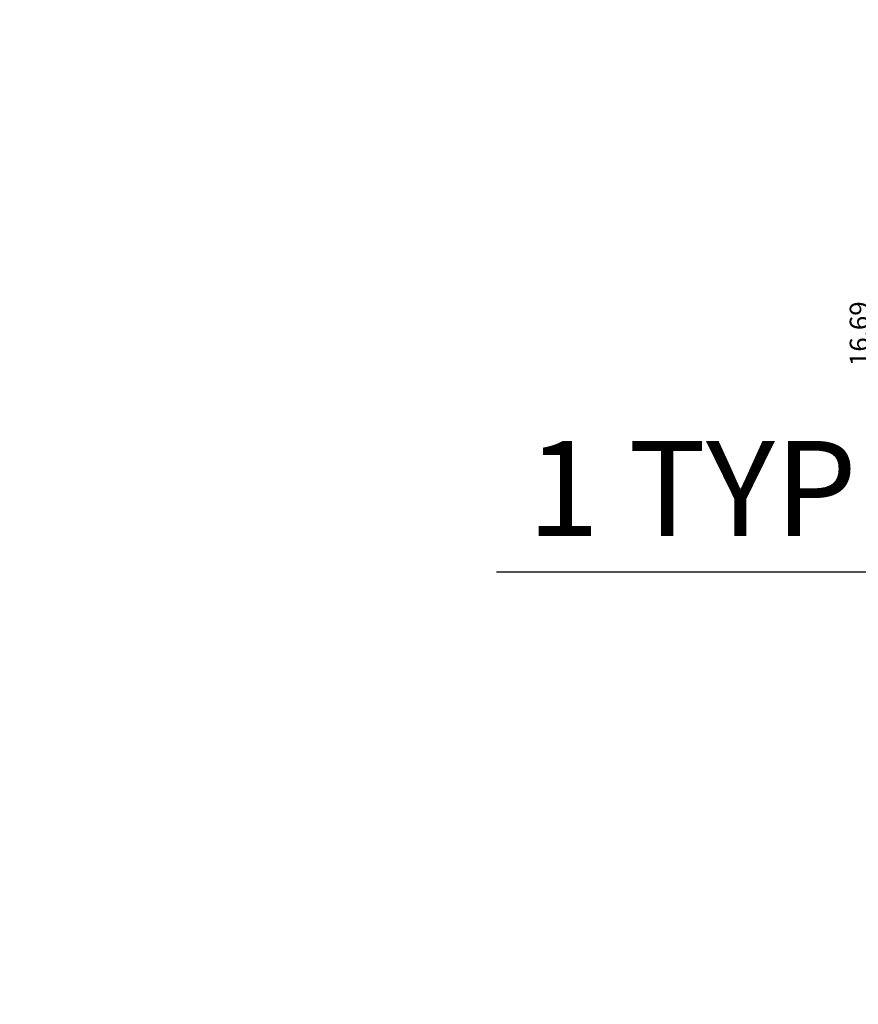
# Model space of a CAD drawing. Units: metres. Extents: x 1246 to 2549, y 2050 to 4184.
# Tile 2 of 6: x 1246 to 1268, y 2074 to 2100. Entities that reach past the tile are written whole.
import ezdxf

# ---------------------------------------------------------------- set-up
doc = ezdxf.new("R2010")
doc.units = ezdxf.units.M
doc.layers.add('A-ANNO-DIMS', color=2, linetype='Continuous', lineweight=18)
doc.styles.get("Standard").update_dxf_attribs({"font": 'arial.ttf'})
doc.dimstyles.new('ISO-25', dxfattribs={"dimtxt": 2.5, "dimasz": 2.5, "dimexe": 1.25, "dimexo": 0.625, "dimtad": 1, "dimtxsty": 'Standard', "dimcen": 2.5, "dimadec": 0, "dimazin": 0, "dimtfac": 1, "dimtmove": 0, "dimatfit": 3, "dimfxl": 1, "dimarcsym": 0})

# ---------------------------------------------------------------- blocks, each defined once
blk = doc.blocks.new('*D2')
at = {"layer": 'A-ANNO-DIMS', "color": 0, "lineweight": -2, "transparency": 16777216}
for p, q in [((1272.709, 2100.209), (1270.53, 2100.209)), ((1271.78, 2097.709), (1271.78, 2086.022)), ((1272.709, 2083.522), (1270.53, 2083.522))]:
    blk.add_line(p, q, dxfattribs=at)
at = {"layer": 'A-ANNO-DIMS', "color": 0, "transparency": 16777216}
for points in [[(1271.364, 2097.709), (1272.197, 2097.709), (1271.78, 2100.209)], [(1271.364, 2086.022), (1272.197, 2086.022), (1271.78, 2083.522)]]:
    blk.add_solid(points, dxfattribs=at)
at = {"layer": 'Defpoints', "color": 0, "transparency": 16777216}
for p in [(1273.334, 2100.209), (1271.78, 2083.522), (1273.334, 2083.522)]:
    blk.add_point(p, dxfattribs=at)
at = {"layer": 'A-ANNO-DIMS', "color": 0, "transparency": 16777216, "insert": (1264.522, 2091.865), "char_height": 2.5, "attachment_point": 5, "rotation": 90}
blk.add_mtext('{\\H0.4x;\\P\\H0.5x;\\P\\P\\P\\P\\P\\P\\P 16,69}', dxfattribs=at)
blk = doc.blocks.new('*D7')
at = {"layer": 'A-ANNO-DIMS', "color": 0, "lineweight": -2, "transparency": 16777216}
for p, q in [((1274.837, 2088.031), (1274.837, 2090.531)), ((1274.346, 2085.531), (1273.587, 2085.531)), ((1274.837, 2085.531), (1274.837, 2084.639)), ((1274.346, 2084.639), (1273.587, 2084.639)), ((1274.837, 2082.139), (1274.837, 2049.849))]:
    blk.add_line(p, q, dxfattribs=at)
at = {"layer": 'A-ANNO-DIMS', "color": 0, "transparency": 16777216}
for points in [[(1274.421, 2088.031), (1275.254, 2088.031), (1274.837, 2085.531)], [(1274.421, 2082.139), (1275.254, 2082.139), (1274.837, 2084.639)]]:
    blk.add_solid(points, dxfattribs=at)
at = {"layer": 'Defpoints', "color": 0, "transparency": 16777216}
for p in [(1274.971, 2085.531), (1274.837, 2084.639), (1274.971, 2084.639)]:
    blk.add_point(p, dxfattribs=at)
at = {"layer": 'A-ANNO-DIMS', "color": 0, "transparency": 16777216, "insert": (1272.918, 2064.744), "char_height": 2.5, "attachment_point": 5, "rotation": 90}
blk.add_mtext('DOOR-813 1 TYP.', dxfattribs=at)
blk = doc.blocks.new('*D8')
at = {"layer": 'A-ANNO-DIMS', "color": 0, "lineweight": -2, "transparency": 16777216}
for p, q in [((1274.971, 2086.156), (1274.971, 2086.914)), ((1275.817, 2086.156), (1275.817, 2086.914)), ((1272.471, 2085.664), (1258.73, 2085.664)), ((1275.817, 2085.664), (1274.971, 2085.664)), ((1278.317, 2085.664), (1280.817, 2085.664))]:
    blk.add_line(p, q, dxfattribs=at)
at = {"layer": 'A-ANNO-DIMS', "color": 0, "transparency": 16777216}
for points in [[(1272.471, 2086.081), (1272.471, 2085.248), (1274.971, 2085.664)], [(1278.317, 2086.081), (1278.317, 2085.248), (1275.817, 2085.664)]]:
    blk.add_solid(points, dxfattribs=at)
at = {"layer": 'Defpoints', "color": 0, "transparency": 16777216}
for p in [(1274.971, 2085.664), (1274.971, 2085.531), (1275.817, 2085.531)]:
    blk.add_point(p, dxfattribs=at)
at = {"layer": 'A-ANNO-DIMS', "color": 0, "transparency": 16777216, "insert": (1264.35, 2087.545), "char_height": 2.5, "attachment_point": 5}
blk.add_mtext('1 TYP.', dxfattribs=at)

msp = doc.modelspace()

# ---------------------------------------------------------------- dimensions: what is measured, and where the dimension line sits
at = {"layer": 'A-ANNO-DIMS'}
for base, p1, p2, angle, text, override, picture, middle in [((1271.7804, 2083.5216), (1273.334, 2100.2088), (1273.334, 2083.5216), 90, '{\\H0.4x;\\P\\H0.5x;\\P\\P\\P\\P\\P\\P\\P <>}', {"dimclrd": 0, "dimclre": 0, "dimclrt": 0}, '*D2', (1264.5216, 2091.8652)), ((1274.971, 2085.6644), (1275.8169, 2085.5308), (1274.971, 2085.5308), 180, '<> TYP.', {"dimdec": 0, "dimlfac": 1, "dimrnd": 0, "dimzin": 0, "dimdsep": 46, "dimlunit": 2}, '*D8', (1264.3503, 2087.5454)), ((1274.8373, 2084.6395), (1274.971, 2085.5308), (1274.971, 2084.6395), 270, 'DOOR-813 <> TYP.', {"dimdec": 0, "dimlfac": 1, "dimrnd": 0, "dimzin": 0, "dimdsep": 46, "dimlunit": 2}, '*D7', (1272.918, 2064.7444))]:
    dim = msp.add_linear_dim(base=base, p1=p1, p2=p2, angle=angle, text=text, dimstyle='ISO-25', override=override, dxfattribs=at)
    dim.commit()
    dim.dimension.update_dxf_attribs({"geometry": picture, "text_midpoint": middle})

doc.saveas('drawing.dxf')
